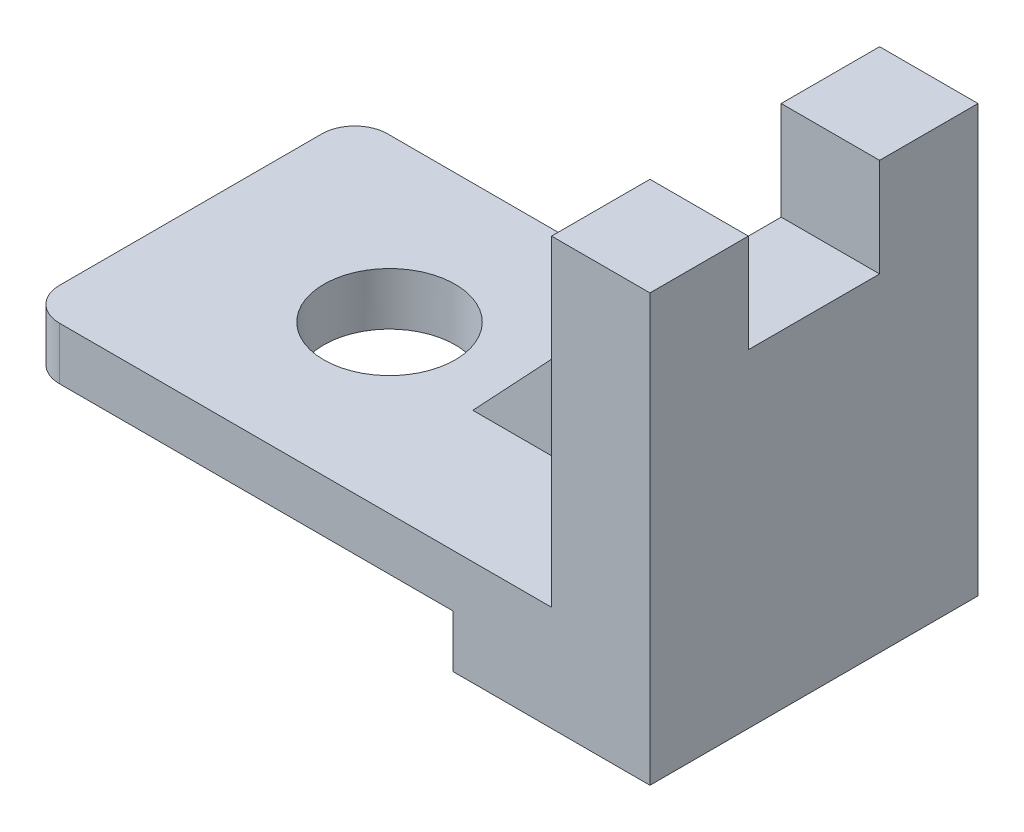
ISO-10303-21;
HEADER;
FILE_DESCRIPTION(('STEP AP214'),'2;1');
FILE_NAME('part.step','',(''),(''),'','','');
FILE_SCHEMA(('AUTOMOTIVE_DESIGN { 1 0 10303 214 1 1 1 1 }'));
ENDSEC;
DATA;
#1=APPLICATION_CONTEXT('core data for automotive mechanical design processes');
#2=APPLICATION_PROTOCOL_DEFINITION('international standard','automotive_design',2000,#1);
#3=PRODUCT_CONTEXT('',#1,'mechanical');
#4=PRODUCT('Part','Part','',(#3));
#5=PRODUCT_RELATED_PRODUCT_CATEGORY('part','',(#4));
#6=PRODUCT_DEFINITION_FORMATION('','',#4);
#7=PRODUCT_DEFINITION_CONTEXT('part definition',#1,'design');
#8=PRODUCT_DEFINITION('design','',#6,#7);
#9=PRODUCT_DEFINITION_SHAPE('','',#8);
#10=(LENGTH_UNIT() NAMED_UNIT(*) SI_UNIT(.MILLI.,.METRE.));
#11=(NAMED_UNIT(*) PLANE_ANGLE_UNIT() SI_UNIT($,.RADIAN.));
#12=(NAMED_UNIT(*) SI_UNIT($,.STERADIAN.) SOLID_ANGLE_UNIT());
#13=UNCERTAINTY_MEASURE_WITH_UNIT(LENGTH_MEASURE(1.E-05),#10,'distance_accuracy_value','');
#14=(GEOMETRIC_REPRESENTATION_CONTEXT(3) GLOBAL_UNCERTAINTY_ASSIGNED_CONTEXT((#13)) GLOBAL_UNIT_ASSIGNED_CONTEXT((#10,
#11,#12)) REPRESENTATION_CONTEXT('',''));
#15=CARTESIAN_POINT('',(0.,0.,0.));
#16=DIRECTION('',(0.,0.,1.));
#17=DIRECTION('',(1.,0.,0.));
#18=AXIS2_PLACEMENT_3D('',#15,#16,#17);
#19=CARTESIAN_POINT('',(-15.,16.,50.));
#20=DIRECTION('',(1.,0.,0.));
#21=DIRECTION('',(0.,0.,-1.));
#22=AXIS2_PLACEMENT_3D('',#19,#20,#21);
#23=PLANE('',#22);
#24=DIRECTION('',(0.,-1.,0.));
#25=VECTOR('',#24,1.);
#26=CARTESIAN_POINT('',(-15.,16.,20.));
#27=LINE('',#26,#25);
#28=CARTESIAN_POINT('',(-15.,50.,20.));
#29=VERTEX_POINT('',#28);
#30=CARTESIAN_POINT('',(-15.,16.,20.));
#31=VERTEX_POINT('',#30);
#32=EDGE_CURVE('E159',#29,#31,#27,.T.);
#33=ORIENTED_EDGE('',*,*,#32,.F.);
#34=DIRECTION('',(0.,0.,1.));
#35=VECTOR('',#34,1.);
#36=CARTESIAN_POINT('',(-15.,50.,35.));
#37=LINE('',#36,#35);
#38=CARTESIAN_POINT('',(-15.,50.,15.));
#39=VERTEX_POINT('',#38);
#40=EDGE_CURVE('E323',#39,#29,#37,.T.);
#41=ORIENTED_EDGE('',*,*,#40,.F.);
#42=DIRECTION('',(0.,1.,0.));
#43=VECTOR('',#42,1.);
#44=CARTESIAN_POINT('',(-15.,50.,15.));
#45=LINE('',#44,#43);
#46=CARTESIAN_POINT('',(-15.,65.,15.));
#47=VERTEX_POINT('',#46);
#48=EDGE_CURVE('E309',#39,#47,#45,.T.);
#49=ORIENTED_EDGE('',*,*,#48,.T.);
#50=DIRECTION('',(0.,0.,-1.));
#51=VECTOR('',#50,1.);
#52=CARTESIAN_POINT('',(-15.,65.,50.));
#53=LINE('',#52,#51);
#54=CARTESIAN_POINT('',(-15.,65.,0.));
#55=VERTEX_POINT('',#54);
#56=EDGE_CURVE('E190',#47,#55,#53,.T.);
#57=ORIENTED_EDGE('',*,*,#56,.T.);
#58=DIRECTION('',(0.,-1.,0.));
#59=VECTOR('',#58,1.);
#60=CARTESIAN_POINT('',(-15.,16.,0.));
#61=LINE('',#60,#59);
#62=CARTESIAN_POINT('',(-15.,16.,0.));
#63=VERTEX_POINT('',#62);
#64=EDGE_CURVE('E185',#55,#63,#61,.T.);
#65=ORIENTED_EDGE('',*,*,#64,.T.);
#66=DIRECTION('',(0.,0.,-1.));
#67=VECTOR('',#66,1.);
#68=CARTESIAN_POINT('',(-15.,16.,50.));
#69=LINE('',#68,#67);
#70=EDGE_CURVE('E177',#31,#63,#69,.T.);
#71=ORIENTED_EDGE('',*,*,#70,.F.);
#72=EDGE_LOOP('',(#33,#41,#49,#57,#65,#71));
#73=FACE_BOUND('',#72,.T.);
#74=ADVANCED_FACE('F39',(#73),#23,.F.);
#75=CARTESIAN_POINT('',(-95.,16.,50.));
#76=DIRECTION('',(0.,-1.,0.));
#77=DIRECTION('',(0.,0.,-1.));
#78=AXIS2_PLACEMENT_3D('',#75,#76,#77);
#79=PLANE('',#78);
#80=CARTESIAN_POINT('',(-65.,16.,24.70063975312));
#81=DIRECTION('',(0.,1.,0.));
#82=DIRECTION('',(0.,0.,1.));
#83=AXIS2_PLACEMENT_3D('',#80,#81,#82);
#84=CIRCLE('',#83,9.99999999999999);
#85=CARTESIAN_POINT('',(-65.,16.,34.70063975312));
#86=VERTEX_POINT('',#85);
#87=EDGE_CURVE('E205',#86,#86,#84,.T.);
#88=ORIENTED_EDGE('',*,*,#87,.F.);
#89=EDGE_LOOP('',(#88));
#90=FACE_BOUND('',#89,.T.);
#91=DIRECTION('',(-1.,0.,0.));
#92=VECTOR('',#91,1.);
#93=CARTESIAN_POINT('',(-15.,16.,20.));
#94=LINE('',#93,#92);
#95=CARTESIAN_POINT('',(-47.,16.,20.));
#96=VERTEX_POINT('',#95);
#97=EDGE_CURVE('E162',#31,#96,#94,.T.);
#98=ORIENTED_EDGE('',*,*,#97,.F.);
#99=ORIENTED_EDGE('',*,*,#70,.T.);
#100=DIRECTION('',(-1.,0.,0.));
#101=VECTOR('',#100,1.);
#102=CARTESIAN_POINT('',(-95.,16.,0.));
#103=LINE('',#102,#101);
#104=CARTESIAN_POINT('',(-90.,16.,0.));
#105=VERTEX_POINT('',#104);
#106=EDGE_CURVE('E212',#63,#105,#103,.T.);
#107=ORIENTED_EDGE('',*,*,#106,.T.);
#108=CARTESIAN_POINT('',(-90.,16.,5.));
#109=DIRECTION('',(0.,-1.,0.));
#110=DIRECTION('',(0.,0.,-1.));
#111=AXIS2_PLACEMENT_3D('',#108,#109,#110);
#112=CIRCLE('',#111,5.);
#113=CARTESIAN_POINT('',(-95.,16.,5.));
#114=VERTEX_POINT('',#113);
#115=EDGE_CURVE('E50',#105,#114,#112,.F.);
#116=ORIENTED_EDGE('',*,*,#115,.T.);
#117=DIRECTION('',(0.,0.,-1.));
#118=VECTOR('',#117,1.);
#119=CARTESIAN_POINT('',(-95.,16.,50.));
#120=LINE('',#119,#118);
#121=CARTESIAN_POINT('',(-95.,16.,45.));
#122=VERTEX_POINT('',#121);
#123=EDGE_CURVE('E183',#122,#114,#120,.T.);
#124=ORIENTED_EDGE('',*,*,#123,.F.);
#125=CARTESIAN_POINT('',(-90.,16.,45.));
#126=DIRECTION('',(0.,-1.,0.));
#127=DIRECTION('',(0.,0.,-1.));
#128=AXIS2_PLACEMENT_3D('',#125,#126,#127);
#129=CIRCLE('',#128,5.);
#130=CARTESIAN_POINT('',(-90.,16.,50.));
#131=VERTEX_POINT('',#130);
#132=EDGE_CURVE('E64',#122,#131,#129,.F.);
#133=ORIENTED_EDGE('',*,*,#132,.T.);
#134=DIRECTION('',(-1.,0.,0.));
#135=VECTOR('',#134,1.);
#136=CARTESIAN_POINT('',(-95.,16.,50.));
#137=LINE('',#136,#135);
#138=CARTESIAN_POINT('',(-15.,16.,50.));
#139=VERTEX_POINT('',#138);
#140=EDGE_CURVE('E264',#139,#131,#137,.T.);
#141=ORIENTED_EDGE('',*,*,#140,.F.);
#142=CARTESIAN_POINT('',(-15.,16.,30.));
#143=VERTEX_POINT('',#142);
#144=EDGE_CURVE('E184',#139,#143,#69,.T.);
#145=ORIENTED_EDGE('',*,*,#144,.T.);
#146=DIRECTION('',(-1.,0.,0.));
#147=VECTOR('',#146,1.);
#148=CARTESIAN_POINT('',(-15.,16.,30.));
#149=LINE('',#148,#147);
#150=CARTESIAN_POINT('',(-47.,16.,30.));
#151=VERTEX_POINT('',#150);
#152=EDGE_CURVE('E337',#143,#151,#149,.T.);
#153=ORIENTED_EDGE('',*,*,#152,.T.);
#154=DIRECTION('',(0.,0.,1.));
#155=VECTOR('',#154,1.);
#156=CARTESIAN_POINT('',(-47.,16.,20.));
#157=LINE('',#156,#155);
#158=EDGE_CURVE('E179',#96,#151,#157,.T.);
#159=ORIENTED_EDGE('',*,*,#158,.F.);
#160=EDGE_LOOP('',(#98,#99,#107,#116,#124,#133,#141,#145,#153,#159));
#161=FACE_BOUND('',#160,.T.);
#162=ADVANCED_FACE('F171',(#90,#161),#79,.F.);
#163=CARTESIAN_POINT('',(-15.,65.,50.));
#164=DIRECTION('',(0.,-1.,0.));
#165=DIRECTION('',(0.,0.,-1.));
#166=AXIS2_PLACEMENT_3D('',#163,#164,#165);
#167=PLANE('',#166);
#168=DIRECTION('',(0.,0.,-1.));
#169=VECTOR('',#168,1.);
#170=CARTESIAN_POINT('',(0.,65.,50.));
#171=LINE('',#170,#169);
#172=CARTESIAN_POINT('',(0.,65.,50.));
#173=VERTEX_POINT('',#172);
#174=CARTESIAN_POINT('',(0.,65.,35.));
#175=VERTEX_POINT('',#174);
#176=EDGE_CURVE('E247',#173,#175,#171,.T.);
#177=ORIENTED_EDGE('',*,*,#176,.T.);
#178=DIRECTION('',(1.,0.,0.));
#179=VECTOR('',#178,1.);
#180=CARTESIAN_POINT('',(0.,65.,35.));
#181=LINE('',#180,#179);
#182=CARTESIAN_POINT('',(-15.,65.,35.));
#183=VERTEX_POINT('',#182);
#184=EDGE_CURVE('E320',#183,#175,#181,.T.);
#185=ORIENTED_EDGE('',*,*,#184,.F.);
#186=CARTESIAN_POINT('',(-15.,65.,50.));
#187=VERTEX_POINT('',#186);
#188=EDGE_CURVE('E194',#187,#183,#53,.T.);
#189=ORIENTED_EDGE('',*,*,#188,.F.);
#190=DIRECTION('',(-1.,0.,0.));
#191=VECTOR('',#190,1.);
#192=CARTESIAN_POINT('',(-15.,65.,50.));
#193=LINE('',#192,#191);
#194=EDGE_CURVE('E243',#173,#187,#193,.T.);
#195=ORIENTED_EDGE('',*,*,#194,.F.);
#196=EDGE_LOOP('',(#177,#185,#189,#195));
#197=FACE_BOUND('',#196,.T.);
#198=ADVANCED_FACE('F303',(#197),#167,.F.);
#199=ORIENTED_EDGE('',*,*,#56,.F.);
#200=DIRECTION('',(-1.,0.,0.));
#201=VECTOR('',#200,1.);
#202=CARTESIAN_POINT('',(-15.,65.,15.));
#203=LINE('',#202,#201);
#204=CARTESIAN_POINT('',(0.,65.,15.));
#205=VERTEX_POINT('',#204);
#206=EDGE_CURVE('E319',#205,#47,#203,.T.);
#207=ORIENTED_EDGE('',*,*,#206,.F.);
#208=CARTESIAN_POINT('',(0.,65.,0.));
#209=VERTEX_POINT('',#208);
#210=EDGE_CURVE('E246',#205,#209,#171,.T.);
#211=ORIENTED_EDGE('',*,*,#210,.T.);
#212=DIRECTION('',(-1.,0.,0.));
#213=VECTOR('',#212,1.);
#214=CARTESIAN_POINT('',(-15.,65.,0.));
#215=LINE('',#214,#213);
#216=EDGE_CURVE('E203',#209,#55,#215,.T.);
#217=ORIENTED_EDGE('',*,*,#216,.T.);
#218=EDGE_LOOP('',(#199,#207,#211,#217));
#219=FACE_BOUND('',#218,.T.);
#220=ADVANCED_FACE('F278',(#219),#167,.F.);
#221=CARTESIAN_POINT('',(-15.,50.,30.));
#222=VERTEX_POINT('',#221);
#223=CARTESIAN_POINT('',(-15.,50.,35.));
#224=VERTEX_POINT('',#223);
#225=EDGE_CURVE('E324',#222,#224,#37,.T.);
#226=ORIENTED_EDGE('',*,*,#225,.F.);
#227=DIRECTION('',(0.,-1.,0.));
#228=VECTOR('',#227,1.);
#229=CARTESIAN_POINT('',(-15.,16.,30.));
#230=LINE('',#229,#228);
#231=EDGE_CURVE('E53',#222,#143,#230,.T.);
#232=ORIENTED_EDGE('',*,*,#231,.T.);
#233=ORIENTED_EDGE('',*,*,#144,.F.);
#234=DIRECTION('',(0.,-1.,0.));
#235=VECTOR('',#234,1.);
#236=CARTESIAN_POINT('',(-15.,16.,50.));
#237=LINE('',#236,#235);
#238=EDGE_CURVE('E267',#187,#139,#237,.T.);
#239=ORIENTED_EDGE('',*,*,#238,.F.);
#240=ORIENTED_EDGE('',*,*,#188,.T.);
#241=DIRECTION('',(0.,1.,0.));
#242=VECTOR('',#241,1.);
#243=CARTESIAN_POINT('',(-15.,50.,35.));
#244=LINE('',#243,#242);
#245=EDGE_CURVE('E314',#224,#183,#244,.T.);
#246=ORIENTED_EDGE('',*,*,#245,.F.);
#247=EDGE_LOOP('',(#226,#232,#233,#239,#240,#246));
#248=FACE_BOUND('',#247,.T.);
#249=ADVANCED_FACE('F345',(#248),#23,.F.);
#250=CARTESIAN_POINT('',(-95.,7.99999999999999,50.));
#251=DIRECTION('',(1.,0.,0.));
#252=DIRECTION('',(0.,0.,-1.));
#253=AXIS2_PLACEMENT_3D('',#250,#251,#252);
#254=PLANE('',#253);
#255=ORIENTED_EDGE('',*,*,#123,.T.);
#256=DIRECTION('',(0.,-1.,0.));
#257=VECTOR('',#256,1.);
#258=CARTESIAN_POINT('',(-95.,7.99999999999999,5.));
#259=LINE('',#258,#257);
#260=CARTESIAN_POINT('',(-95.,7.99999999999999,5.));
#261=VERTEX_POINT('',#260);
#262=EDGE_CURVE('E204',#114,#261,#259,.T.);
#263=ORIENTED_EDGE('',*,*,#262,.T.);
#264=DIRECTION('',(0.,0.,-1.));
#265=VECTOR('',#264,1.);
#266=CARTESIAN_POINT('',(-95.,7.99999999999999,50.));
#267=LINE('',#266,#265);
#268=CARTESIAN_POINT('',(-95.,7.99999999999999,45.));
#269=VERTEX_POINT('',#268);
#270=EDGE_CURVE('E188',#269,#261,#267,.T.);
#271=ORIENTED_EDGE('',*,*,#270,.F.);
#272=DIRECTION('',(0.,-1.,0.));
#273=VECTOR('',#272,1.);
#274=CARTESIAN_POINT('',(-95.,7.99999999999999,45.));
#275=LINE('',#274,#273);
#276=EDGE_CURVE('E197',#269,#122,#275,.F.);
#277=ORIENTED_EDGE('',*,*,#276,.T.);
#278=EDGE_LOOP('',(#255,#263,#271,#277));
#279=FACE_BOUND('',#278,.T.);
#280=ADVANCED_FACE('F218',(#279),#254,.F.);
#281=CARTESIAN_POINT('',(-30.,8.,50.));
#282=DIRECTION('',(0.,1.,0.));
#283=DIRECTION('',(-1.,0.,0.));
#284=AXIS2_PLACEMENT_3D('',#281,#282,#283);
#285=PLANE('',#284);
#286=CARTESIAN_POINT('',(-65.,7.99999999999999,24.70063975312));
#287=DIRECTION('',(0.,1.,0.));
#288=DIRECTION('',(-1.,0.,0.));
#289=AXIS2_PLACEMENT_3D('',#286,#287,#288);
#290=CIRCLE('',#289,9.99999999999999);
#291=CARTESIAN_POINT('',(-75.,7.99999999999998,24.70063975312));
#292=VERTEX_POINT('',#291);
#293=EDGE_CURVE('E196',#292,#292,#290,.T.);
#294=ORIENTED_EDGE('',*,*,#293,.T.);
#295=EDGE_LOOP('',(#294));
#296=FACE_BOUND('',#295,.T.);
#297=ORIENTED_EDGE('',*,*,#270,.T.);
#298=CARTESIAN_POINT('',(-90.,7.99999999999999,5.));
#299=DIRECTION('',(0.,1.,0.));
#300=DIRECTION('',(-1.,0.,0.));
#301=AXIS2_PLACEMENT_3D('',#298,#299,#300);
#302=CIRCLE('',#301,5.);
#303=CARTESIAN_POINT('',(-90.,7.99999999999999,0.));
#304=VERTEX_POINT('',#303);
#305=EDGE_CURVE('E207',#261,#304,#302,.F.);
#306=ORIENTED_EDGE('',*,*,#305,.T.);
#307=DIRECTION('',(1.,0.,0.));
#308=VECTOR('',#307,1.);
#309=CARTESIAN_POINT('',(-30.,8.,0.));
#310=LINE('',#309,#308);
#311=CARTESIAN_POINT('',(-30.,8.,0.));
#312=VERTEX_POINT('',#311);
#313=EDGE_CURVE('E230',#304,#312,#310,.T.);
#314=ORIENTED_EDGE('',*,*,#313,.T.);
#315=DIRECTION('',(0.,0.,-1.));
#316=VECTOR('',#315,1.);
#317=CARTESIAN_POINT('',(-30.,8.,50.));
#318=LINE('',#317,#316);
#319=CARTESIAN_POINT('',(-30.,8.,50.));
#320=VERTEX_POINT('',#319);
#321=EDGE_CURVE('E258',#320,#312,#318,.T.);
#322=ORIENTED_EDGE('',*,*,#321,.F.);
#323=DIRECTION('',(1.,0.,0.));
#324=VECTOR('',#323,1.);
#325=CARTESIAN_POINT('',(-30.,8.,50.));
#326=LINE('',#325,#324);
#327=CARTESIAN_POINT('',(-90.,7.99999999999999,50.));
#328=VERTEX_POINT('',#327);
#329=EDGE_CURVE('E263',#328,#320,#326,.T.);
#330=ORIENTED_EDGE('',*,*,#329,.F.);
#331=CARTESIAN_POINT('',(-90.,7.99999999999999,45.));
#332=DIRECTION('',(0.,1.,0.));
#333=DIRECTION('',(-1.,0.,0.));
#334=AXIS2_PLACEMENT_3D('',#331,#332,#333);
#335=CIRCLE('',#334,5.);
#336=EDGE_CURVE('E210',#328,#269,#335,.F.);
#337=ORIENTED_EDGE('',*,*,#336,.T.);
#338=EDGE_LOOP('',(#297,#306,#314,#322,#330,#337));
#339=FACE_BOUND('',#338,.T.);
#340=ADVANCED_FACE('F227',(#296,#339),#285,.F.);
#341=CARTESIAN_POINT('',(-30.,0.,50.));
#342=DIRECTION('',(1.,0.,0.));
#343=DIRECTION('',(0.,0.,-1.));
#344=AXIS2_PLACEMENT_3D('',#341,#342,#343);
#345=PLANE('',#344);
#346=DIRECTION('',(0.,-1.,0.));
#347=VECTOR('',#346,1.);
#348=CARTESIAN_POINT('',(-30.,0.,0.));
#349=LINE('',#348,#347);
#350=CARTESIAN_POINT('',(-30.,0.,0.));
#351=VERTEX_POINT('',#350);
#352=EDGE_CURVE('E234',#312,#351,#349,.T.);
#353=ORIENTED_EDGE('',*,*,#352,.T.);
#354=DIRECTION('',(0.,0.,-1.));
#355=VECTOR('',#354,1.);
#356=CARTESIAN_POINT('',(-30.,0.,50.));
#357=LINE('',#356,#355);
#358=CARTESIAN_POINT('',(-30.,0.,50.));
#359=VERTEX_POINT('',#358);
#360=EDGE_CURVE('E251',#359,#351,#357,.T.);
#361=ORIENTED_EDGE('',*,*,#360,.F.);
#362=DIRECTION('',(0.,-1.,0.));
#363=VECTOR('',#362,1.);
#364=CARTESIAN_POINT('',(-30.,0.,50.));
#365=LINE('',#364,#363);
#366=EDGE_CURVE('E261',#320,#359,#365,.T.);
#367=ORIENTED_EDGE('',*,*,#366,.F.);
#368=ORIENTED_EDGE('',*,*,#321,.T.);
#369=EDGE_LOOP('',(#353,#361,#367,#368));
#370=FACE_BOUND('',#369,.T.);
#371=ADVANCED_FACE('F259',(#370),#345,.F.);
#372=CARTESIAN_POINT('',(0.,0.,50.));
#373=DIRECTION('',(0.,1.,0.));
#374=DIRECTION('',(0.,0.,1.));
#375=AXIS2_PLACEMENT_3D('',#372,#373,#374);
#376=PLANE('',#375);
#377=DIRECTION('',(1.,0.,0.));
#378=VECTOR('',#377,1.);
#379=CARTESIAN_POINT('',(0.,0.,0.));
#380=LINE('',#379,#378);
#381=CARTESIAN_POINT('',(0.,0.,0.));
#382=VERTEX_POINT('',#381);
#383=EDGE_CURVE('E237',#351,#382,#380,.T.);
#384=ORIENTED_EDGE('',*,*,#383,.T.);
#385=DIRECTION('',(0.,0.,-1.));
#386=VECTOR('',#385,1.);
#387=CARTESIAN_POINT('',(0.,0.,50.));
#388=LINE('',#387,#386);
#389=CARTESIAN_POINT('',(0.,0.,50.));
#390=VERTEX_POINT('',#389);
#391=EDGE_CURVE('E249',#390,#382,#388,.T.);
#392=ORIENTED_EDGE('',*,*,#391,.F.);
#393=DIRECTION('',(1.,0.,0.));
#394=VECTOR('',#393,1.);
#395=CARTESIAN_POINT('',(0.,0.,50.));
#396=LINE('',#395,#394);
#397=EDGE_CURVE('E270',#359,#390,#396,.T.);
#398=ORIENTED_EDGE('',*,*,#397,.F.);
#399=ORIENTED_EDGE('',*,*,#360,.T.);
#400=EDGE_LOOP('',(#384,#392,#398,#399));
#401=FACE_BOUND('',#400,.T.);
#402=ADVANCED_FACE('F291',(#401),#376,.F.);
#403=CARTESIAN_POINT('',(0.,65.,50.));
#404=DIRECTION('',(-1.,0.,0.));
#405=DIRECTION('',(0.,-1.,0.));
#406=AXIS2_PLACEMENT_3D('',#403,#404,#405);
#407=PLANE('',#406);
#408=DIRECTION('',(0.,0.,-1.));
#409=VECTOR('',#408,1.);
#410=CARTESIAN_POINT('',(0.,50.,15.));
#411=LINE('',#410,#409);
#412=CARTESIAN_POINT('',(0.,50.,35.));
#413=VERTEX_POINT('',#412);
#414=CARTESIAN_POINT('',(0.,50.,15.));
#415=VERTEX_POINT('',#414);
#416=EDGE_CURVE('E317',#413,#415,#411,.T.);
#417=ORIENTED_EDGE('',*,*,#416,.F.);
#418=DIRECTION('',(0.,1.,0.));
#419=VECTOR('',#418,1.);
#420=CARTESIAN_POINT('',(0.,50.,35.));
#421=LINE('',#420,#419);
#422=EDGE_CURVE('E298',#413,#175,#421,.T.);
#423=ORIENTED_EDGE('',*,*,#422,.T.);
#424=ORIENTED_EDGE('',*,*,#176,.F.);
#425=DIRECTION('',(0.,1.,0.));
#426=VECTOR('',#425,1.);
#427=CARTESIAN_POINT('',(0.,65.,50.));
#428=LINE('',#427,#426);
#429=EDGE_CURVE('E273',#390,#173,#428,.T.);
#430=ORIENTED_EDGE('',*,*,#429,.F.);
#431=ORIENTED_EDGE('',*,*,#391,.T.);
#432=DIRECTION('',(0.,1.,0.));
#433=VECTOR('',#432,1.);
#434=CARTESIAN_POINT('',(0.,65.,0.));
#435=LINE('',#434,#433);
#436=EDGE_CURVE('E244',#382,#209,#435,.T.);
#437=ORIENTED_EDGE('',*,*,#436,.T.);
#438=ORIENTED_EDGE('',*,*,#210,.F.);
#439=DIRECTION('',(0.,1.,0.));
#440=VECTOR('',#439,1.);
#441=CARTESIAN_POINT('',(0.,50.,15.));
#442=LINE('',#441,#440);
#443=EDGE_CURVE('E306',#415,#205,#442,.T.);
#444=ORIENTED_EDGE('',*,*,#443,.F.);
#445=EDGE_LOOP('',(#417,#423,#424,#430,#431,#437,#438,#444));
#446=FACE_BOUND('',#445,.T.);
#447=ADVANCED_FACE('F287',(#446),#407,.F.);
#448=CARTESIAN_POINT('',(0.,0.,50.));
#449=DIRECTION('',(0.,0.,-1.));
#450=DIRECTION('',(-1.,0.,0.));
#451=AXIS2_PLACEMENT_3D('',#448,#449,#450);
#452=PLANE('',#451);
#453=ORIENTED_EDGE('',*,*,#140,.T.);
#454=DIRECTION('',(0.,-1.,0.));
#455=VECTOR('',#454,1.);
#456=CARTESIAN_POINT('',(-90.,0.,50.));
#457=LINE('',#456,#455);
#458=EDGE_CURVE('E11',#131,#328,#457,.T.);
#459=ORIENTED_EDGE('',*,*,#458,.T.);
#460=ORIENTED_EDGE('',*,*,#329,.T.);
#461=ORIENTED_EDGE('',*,*,#366,.T.);
#462=ORIENTED_EDGE('',*,*,#397,.T.);
#463=ORIENTED_EDGE('',*,*,#429,.T.);
#464=ORIENTED_EDGE('',*,*,#194,.T.);
#465=ORIENTED_EDGE('',*,*,#238,.T.);
#466=EDGE_LOOP('',(#453,#459,#460,#461,#462,#463,#464,#465));
#467=FACE_BOUND('',#466,.T.);
#468=ADVANCED_FACE('F294',(#467),#452,.F.);
#469=CARTESIAN_POINT('',(0.,0.,0.));
#470=DIRECTION('',(0.,0.,-1.));
#471=DIRECTION('',(-1.,0.,0.));
#472=AXIS2_PLACEMENT_3D('',#469,#470,#471);
#473=PLANE('',#472);
#474=ORIENTED_EDGE('',*,*,#313,.F.);
#475=DIRECTION('',(0.,-1.,0.));
#476=VECTOR('',#475,1.);
#477=CARTESIAN_POINT('',(-90.,16.,0.));
#478=LINE('',#477,#476);
#479=EDGE_CURVE('E211',#304,#105,#478,.F.);
#480=ORIENTED_EDGE('',*,*,#479,.T.);
#481=ORIENTED_EDGE('',*,*,#106,.F.);
#482=ORIENTED_EDGE('',*,*,#64,.F.);
#483=ORIENTED_EDGE('',*,*,#216,.F.);
#484=ORIENTED_EDGE('',*,*,#436,.F.);
#485=ORIENTED_EDGE('',*,*,#383,.F.);
#486=ORIENTED_EDGE('',*,*,#352,.F.);
#487=EDGE_LOOP('',(#474,#480,#481,#482,#483,#484,#485,#486));
#488=FACE_BOUND('',#487,.T.);
#489=ADVANCED_FACE('F235',(#488),#473,.T.);
#490=CARTESIAN_POINT('',(-65.,-34.,24.70063975312));
#491=DIRECTION('',(0.,1.,0.));
#492=DIRECTION('',(0.,0.,1.));
#493=AXIS2_PLACEMENT_3D('',#490,#491,#492);
#494=CYLINDRICAL_SURFACE('',#493,9.99999999999999);
#495=ORIENTED_EDGE('',*,*,#87,.T.);
#496=EDGE_LOOP('',(#495));
#497=FACE_BOUND('',#496,.T.);
#498=ORIENTED_EDGE('',*,*,#293,.F.);
#499=EDGE_LOOP('',(#498));
#500=FACE_BOUND('',#499,.T.);
#501=ADVANCED_FACE('F381',(#497,#500),#494,.F.);
#502=CARTESIAN_POINT('',(0.,50.,35.));
#503=DIRECTION('',(0.,0.,1.));
#504=DIRECTION('',(1.,0.,0.));
#505=AXIS2_PLACEMENT_3D('',#502,#503,#504);
#506=PLANE('',#505);
#507=ORIENTED_EDGE('',*,*,#184,.T.);
#508=ORIENTED_EDGE('',*,*,#422,.F.);
#509=DIRECTION('',(1.,0.,0.));
#510=VECTOR('',#509,1.);
#511=CARTESIAN_POINT('',(0.,50.,35.));
#512=LINE('',#511,#510);
#513=EDGE_CURVE('E313',#224,#413,#512,.T.);
#514=ORIENTED_EDGE('',*,*,#513,.F.);
#515=ORIENTED_EDGE('',*,*,#245,.T.);
#516=EDGE_LOOP('',(#507,#508,#514,#515));
#517=FACE_BOUND('',#516,.T.);
#518=ADVANCED_FACE('F384',(#517),#506,.F.);
#519=CARTESIAN_POINT('',(-15.,50.,15.));
#520=DIRECTION('',(0.,0.,-1.));
#521=DIRECTION('',(-1.,0.,0.));
#522=AXIS2_PLACEMENT_3D('',#519,#520,#521);
#523=PLANE('',#522);
#524=ORIENTED_EDGE('',*,*,#206,.T.);
#525=ORIENTED_EDGE('',*,*,#48,.F.);
#526=DIRECTION('',(-1.,0.,0.));
#527=VECTOR('',#526,1.);
#528=CARTESIAN_POINT('',(-15.,50.,15.));
#529=LINE('',#528,#527);
#530=EDGE_CURVE('E326',#415,#39,#529,.T.);
#531=ORIENTED_EDGE('',*,*,#530,.F.);
#532=ORIENTED_EDGE('',*,*,#443,.T.);
#533=EDGE_LOOP('',(#524,#525,#531,#532));
#534=FACE_BOUND('',#533,.T.);
#535=ADVANCED_FACE('F431',(#534),#523,.F.);
#536=CARTESIAN_POINT('',(0.,50.,0.));
#537=DIRECTION('',(0.,-1.,0.));
#538=DIRECTION('',(0.,0.,-1.));
#539=AXIS2_PLACEMENT_3D('',#536,#537,#538);
#540=PLANE('',#539);
#541=ORIENTED_EDGE('',*,*,#416,.T.);
#542=ORIENTED_EDGE('',*,*,#530,.T.);
#543=ORIENTED_EDGE('',*,*,#40,.T.);
#544=DIRECTION('',(0.,0.,1.));
#545=VECTOR('',#544,1.);
#546=CARTESIAN_POINT('',(-15.,50.,20.));
#547=LINE('',#546,#545);
#548=EDGE_CURVE('E335',#29,#222,#547,.T.);
#549=ORIENTED_EDGE('',*,*,#548,.T.);
#550=ORIENTED_EDGE('',*,*,#225,.T.);
#551=ORIENTED_EDGE('',*,*,#513,.T.);
#552=EDGE_LOOP('',(#541,#542,#543,#549,#550,#551));
#553=FACE_BOUND('',#552,.T.);
#554=ADVANCED_FACE('F353',(#553),#540,.F.);
#555=CARTESIAN_POINT('',(-90.,7.99999999999999,5.));
#556=DIRECTION('',(0.,1.,0.));
#557=DIRECTION('',(0.,0.,1.));
#558=AXIS2_PLACEMENT_3D('',#555,#556,#557);
#559=CYLINDRICAL_SURFACE('',#558,5.);
#560=ORIENTED_EDGE('',*,*,#115,.F.);
#561=ORIENTED_EDGE('',*,*,#479,.F.);
#562=ORIENTED_EDGE('',*,*,#305,.F.);
#563=ORIENTED_EDGE('',*,*,#262,.F.);
#564=EDGE_LOOP('',(#560,#561,#562,#563));
#565=FACE_BOUND('',#564,.T.);
#566=ADVANCED_FACE('F224',(#565),#559,.T.);
#567=CARTESIAN_POINT('',(-90.,0.,45.));
#568=DIRECTION('',(0.,-1.,0.));
#569=DIRECTION('',(0.,0.,-1.));
#570=AXIS2_PLACEMENT_3D('',#567,#568,#569);
#571=CYLINDRICAL_SURFACE('',#570,5.);
#572=ORIENTED_EDGE('',*,*,#132,.F.);
#573=ORIENTED_EDGE('',*,*,#276,.F.);
#574=ORIENTED_EDGE('',*,*,#336,.F.);
#575=ORIENTED_EDGE('',*,*,#458,.F.);
#576=EDGE_LOOP('',(#572,#573,#574,#575));
#577=FACE_BOUND('',#576,.T.);
#578=ADVANCED_FACE('F41',(#577),#571,.T.);
#579=CARTESIAN_POINT('',(-15.,50.,20.));
#580=DIRECTION('',(0.728199992692803,-0.685364699004991,0.));
#581=DIRECTION('',(0.685364699004991,0.728199992692803,0.));
#582=AXIS2_PLACEMENT_3D('',#579,#580,#581);
#583=PLANE('',#582);
#584=DIRECTION('',(0.685364699004991,0.728199992692803,0.));
#585=VECTOR('',#584,1.);
#586=CARTESIAN_POINT('',(-15.,50.,30.));
#587=LINE('',#586,#585);
#588=EDGE_CURVE('E172',#151,#222,#587,.T.);
#589=ORIENTED_EDGE('',*,*,#588,.T.);
#590=ORIENTED_EDGE('',*,*,#548,.F.);
#591=DIRECTION('',(0.685364699004991,0.728199992692803,0.));
#592=VECTOR('',#591,1.);
#593=CARTESIAN_POINT('',(-15.,50.,20.));
#594=LINE('',#593,#592);
#595=EDGE_CURVE('E164',#96,#29,#594,.T.);
#596=ORIENTED_EDGE('',*,*,#595,.F.);
#597=ORIENTED_EDGE('',*,*,#158,.T.);
#598=EDGE_LOOP('',(#589,#590,#596,#597));
#599=FACE_BOUND('',#598,.T.);
#600=ADVANCED_FACE('F350',(#599),#583,.F.);
#601=CARTESIAN_POINT('',(0.,0.,20.));
#602=DIRECTION('',(0.,0.,1.));
#603=DIRECTION('',(1.,0.,0.));
#604=AXIS2_PLACEMENT_3D('',#601,#602,#603);
#605=PLANE('',#604);
#606=ORIENTED_EDGE('',*,*,#32,.T.);
#607=ORIENTED_EDGE('',*,*,#97,.T.);
#608=ORIENTED_EDGE('',*,*,#595,.T.);
#609=EDGE_LOOP('',(#606,#607,#608));
#610=FACE_BOUND('',#609,.T.);
#611=ADVANCED_FACE('F165',(#610),#605,.F.);
#612=CARTESIAN_POINT('',(0.,0.,30.));
#613=DIRECTION('',(0.,0.,1.));
#614=DIRECTION('',(1.,0.,0.));
#615=AXIS2_PLACEMENT_3D('',#612,#613,#614);
#616=PLANE('',#615);
#617=ORIENTED_EDGE('',*,*,#231,.F.);
#618=ORIENTED_EDGE('',*,*,#588,.F.);
#619=ORIENTED_EDGE('',*,*,#152,.F.);
#620=EDGE_LOOP('',(#617,#618,#619));
#621=FACE_BOUND('',#620,.T.);
#622=ADVANCED_FACE('F502',(#621),#616,.T.);
#623=CLOSED_SHELL('',(#74,#162,#198,#220,#249,#280,#340,#371,#402,#447,#468,#489,#501,#518,#535,
#554,#566,#578,#600,#611,#622));
#624=MANIFOLD_SOLID_BREP('B2',#623);
#625=ADVANCED_BREP_SHAPE_REPRESENTATION('',(#18,#624),#14);
#626=SHAPE_DEFINITION_REPRESENTATION(#9,#625);
ENDSEC;
END-ISO-10303-21;
